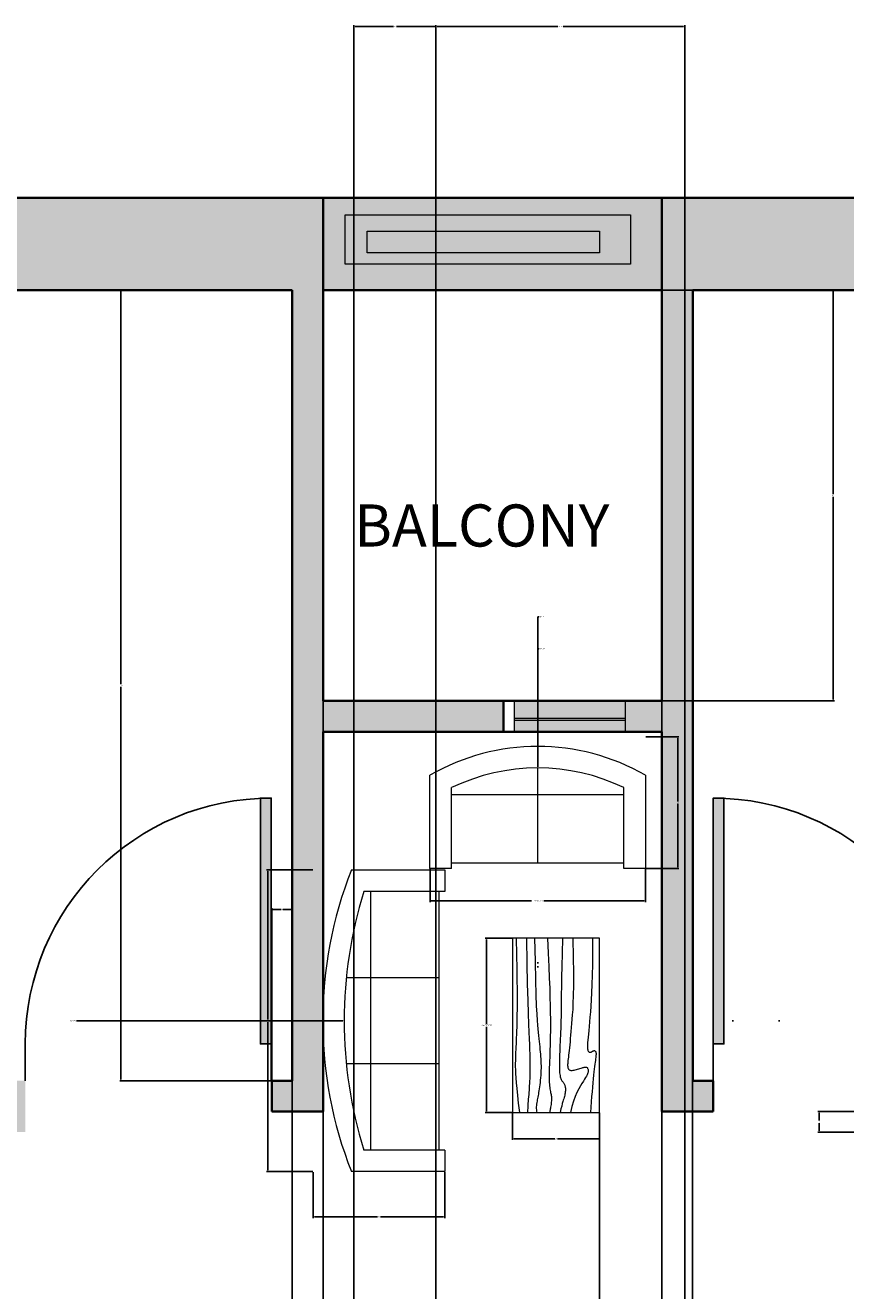
# Model space of a CAD drawing. Units: inches. Extents: x 1434 to 1845, y 1483 to 2014.
# Tile 10 of 11: x 1573 to 1693, y 1829 to 2014. Entities that reach past the tile are written whole.
import ezdxf

# ---------------------------------------------------------------- set-up
doc = ezdxf.new("R2010")
doc.units = ezdxf.units.IN
for name, color, linetype, lineweight in [('A-ANNO-DIMS', 2, 'Continuous', 18), ('A-AREA-IDEN', 7, 'Continuous', 25), ('A-DOOR', 3, 'Continuous', 25), ('A-FURN', 9, 'Continuous', 18), ('A-GLAZ', 4, 'Continuous', 18), ('A-GLAZ-PATT', 9, 'Continuous', 13), ('A-WALL', 7, 'Continuous', 35), ('A-WALL-PATT', 8, 'Continuous', 13)]:
    doc.layers.add(name, color=color, linetype=linetype, lineweight=lineweight)
doc.layers.add('A-DOOR-PATT', color=39, linetype='Continuous', lineweight=13, true_color=0x58382b)
doc.styles.get("Standard").update_dxf_attribs({"font": 'arial.ttf'})
doc.dimstyles.get("Standard").update_dxf_attribs({"dimtxt": 0.18, "dimasz": 0.18, "dimexe": 0.18, "dimexo": 0.0625, "dimgap": 0.09, "dimtad": 0, "dimtih": 1, "dimtoh": 1, "dimdec": 4, "dimzin": 0, "dimdsep": 46, "dimtxsty": 'Standard', "dimcen": 0.09, "dimadec": 0, "dimazin": 0, "dimtfac": 1, "dimtdec": 4, "dimtofl": 0, "dimtmove": 0, "dimatfit": 3, "dimfxl": 1, "dimtolj": 1, "dimtzin": 0, "dimarcsym": 0})

# ---------------------------------------------------------------- blocks, each defined once
blk = doc.blocks.new('*U2')
for p, q in [((0, 0), (0, -6)), ((-40, 0), (-40, -6))]:
    blk.add_line(p, q)
blk.add_lwpolyline([(0, 0), (0, 40), (-1.75, 40), (-1.75, 0)], close=True)
blk.add_arc((0, 0), 40, 90, 180)
blk = doc.blocks.new('*U3')
for p, q in [((0, 0), (0, -6)), ((40, 0), (40, -6))]:
    blk.add_line(p, q)
blk.add_lwpolyline([(0, 0), (0, 40), (1.75, 40), (1.75, 0)], close=True)
blk.add_arc((0, 0), 40, 0, 90)
blk = doc.blocks.new('Sofa - Roundback 7 ft.')
for p, q in [((-12.00002, -32.4421), (-12.00003, -6.5971)), ((11.99997, -32.4421), (11.99998, -6.5971)), ((-36.000027, -34), (-36.000027, -11.4696)), ((-35.999844, -13.3819), (35.9998, -13.3819)), ((35.99998, -34), (35.99998, -11.4696)), ((-36.000027, -32.4421), (35.99998, -32.4421))]:
    blk.add_line(p, q)
for points in [[(-36.000027, -34), (-42.000027, -34), (-42.000027, -8)], [(41.99998, -8), (41.99998, -34), (35.99998, -34)]]:
    blk.add_lwpolyline(points)
for centre, radius, start, end in [((0, -114.25), 114.25, 68.43141, 111.5686), ((-0.00001, -127.1968), 121.1968, 72.72033, 107.2797)]:
    blk.add_arc(centre, radius, start, end)
blk = doc.blocks.new('Sofa - Roundback Loveseat 5 ft.')
for p, q in [((0, -32.44198), (0, -5.99998)), ((-24, -33.99998), (-24, -11.46958)), ((-23.9998, -13.38178), (23.99986, -13.38178)), ((24.00004, -33.99998), (24.00004, -11.46958)), ((-24, -32.44198), (24.00004, -32.44198))]:
    blk.add_line(p, q)
for points in [[(-24, -33.99998), (-30, -33.99998), (-30, -7.99998)], [(30.00004, -7.99998), (30.00004, -33.99998), (24.00004, -33.99998)]]:
    blk.add_lwpolyline(points)
for centre, radius, start, end in [((0, -60.24998), 60.24998, 60.13715, 119.8628), ((0, -61.38438), 55.38444, 64.32083, 115.6792)]:
    blk.add_arc(centre, radius, start, end)
blk = doc.blocks.new('Table - Rectangular Woodgrain 60 x 30 in.')
for p, q in [((0, 0), (0, -30)), ((60, 0), (0, 0)), ((60, -30), (60, 0)), ((0, -30), (60, -30))]:
    blk.add_line(p, q)
for points in [[(0, -2.4), (4.8155, -2.418), (9.0302, -2.4688), (12.709, -2.5477), (15.9167, -2.65), (18.7181, -2.7711), (21.1781, -2.9063), (23.3616, -3.0508), (25.3333, -3.2), (27.1477, -3.3495), (28.8172, -3.4958), (30.3437, -3.636), (31.7291, -3.7667), (32.9756, -3.8849), (34.0849, -3.9875), (35.059, -4.0714), (35.9, -4.1334), (36.6114, -4.1711), (37.2041, -4.1854), (37.6906, -4.1779), (38.0833, -4.15), (38.3948, -4.1034), (38.6375, -4.0396), (38.8239, -3.9602), (38.9666, -3.8667), (39.0764, -3.7608), (39.1573, -3.6448), (39.2116, -3.521), (39.2416, -3.3917), (39.2498, -3.2593), (39.2385, -3.1261), (39.21, -2.9944), (39.1666, -2.8667), (39.111, -2.7447), (39.0468, -2.6281), (38.978, -2.5163), (38.9083, -2.4083), (38.8418, -2.3035), (38.7823, -2.201), (38.7337, -2.1001), (38.7, -2), (38.6844, -1.9003), (38.6875, -1.8021), (38.7094, -1.707), (38.75, -1.6167), (38.8094, -1.5326), (38.8875, -1.4563), (38.9844, -1.3893), (39.1, -1.3333), (39.2351, -1.2896), (39.3937, -1.2583), (39.5804, -1.2396), (39.8, -1.2333), (40.057, -1.2396), (40.3562, -1.2583), (40.7023, -1.2896), (41.1, -1.3333), (41.5547, -1.3895), (42.0755, -1.4573), (42.6721, -1.5361), (43.3542, -1.625), (44.1316, -1.7233), (45.014, -1.8302), (46.0114, -1.9449), (47.1333, -2.0667), (48.3862, -2.1947), (49.7625, -2.3281), (51.2513, -2.4663), (52.8416, -2.6083), (54.5226, -2.7535), (56.2833, -2.9011), (58.1127, -3.0501), (60, -3.2)], [(0, -9.2), (6.5759, -9.0858), (11.9385, -9.0365), (16.2527, -9.0418), (19.6833, -9.0917), (22.3952, -9.1759), (24.5531, -9.2844), (26.322, -9.4069), (27.8666, -9.5333), (29.3241, -9.6553), (30.7203, -9.7719), (32.0532, -9.8837), (33.3208, -9.9917), (34.5213, -10.0965), (35.6526, -10.199), (36.7128, -10.2999), (37.7, -10.4), (38.6129, -10.4996), (39.4531, -10.5969), (40.223, -10.6895), (40.925, -10.775), (41.5613, -10.8512), (42.1344, -10.9156), (42.6465, -10.966), (43.1, -11), (43.4976, -11.0158), (43.8437, -11.0136), (44.143, -10.9942), (44.4, -10.9583), (44.6195, -10.9069), (44.8062, -10.8406), (44.9648, -10.7603), (45.1, -10.6667), (45.2155, -10.5598), (45.3114, -10.4365), (45.3871, -10.2929), (45.4416, -10.125), (45.4743, -9.929), (45.4844, -9.7011), (45.4709, -9.4371), (45.4333, -9.1333), (45.3716, -8.7883), (45.2896, -8.4104), (45.1919, -8.0107), (45.0833, -7.6), (44.9685, -7.1893), (44.8521, -6.7896), (44.7388, -6.4117), (44.6333, -6.0667), (44.54, -5.7628), (44.4614, -5.4979), (44.4001, -5.2675), (44.3583, -5.0667), (44.3384, -4.8909), (44.3427, -4.7354), (44.3736, -4.5956), (44.4333, -4.4667), (44.5236, -4.3453), (44.6427, -4.2333), (44.7884, -4.1339), (44.9583, -4.05), (45.1501, -3.9849), (45.3614, -3.9417), (45.59, -3.9234), (45.8333, -3.9333), (46.0915, -3.9749), (46.3734, -4.0531), (46.6906, -4.1736), (47.0542, -4.3417), (47.4756, -4.5629), (47.9661, -4.8427), (48.5372, -5.1866), (49.2, -5.6), (49.9676, -6.0844), (50.8594, -6.625), (51.8965, -7.2031), (53.1, -7.8), (54.491, -8.3969), (56.0906, -8.975), (57.9199, -9.5156), (60, -10)], [(0, -12.8), (5.1847, -12.9322), (9.6213, -13.0323), (13.3963, -13.1059), (16.5958, -13.1583), (19.3063, -13.1952), (21.614, -13.2219), (23.6054, -13.2439), (25.3666, -13.2667), (26.9728, -13.2947), (28.4531, -13.3281), (29.8256, -13.3663), (31.1083, -13.4083), (32.3191, -13.4535), (33.476, -13.501), (34.597, -13.5501), (35.7, -13.6), (36.7984, -13.6497), (37.8875, -13.6979), (38.9578, -13.743), (40, -13.7833), (41.0047, -13.8174), (41.9625, -13.8438), (42.864, -13.8607), (43.7, -13.8667), (44.4631, -13.8604), (45.1552, -13.8417), (45.7801, -13.8104), (46.3416, -13.7667), (46.8439, -13.7104), (47.2906, -13.6417), (47.6858, -13.5604), (48.0333, -13.4667), (48.3375, -13.3608), (48.6042, -13.2448), (48.8396, -13.121), (49.05, -12.9917), (49.2417, -12.8593), (49.4208, -12.7261), (49.5937, -12.5944), (49.7667, -12.4667), (49.9452, -12.3451), (50.1323, -12.2313), (50.3303, -12.1268), (50.5416, -12.0333), (50.7686, -11.9524), (51.0135, -11.8854), (51.2788, -11.8341), (51.5666, -11.8), (51.8785, -11.7843), (52.2116, -11.7865), (52.562, -11.8059), (52.926, -11.8417), (53.2998, -11.8931), (53.6795, -11.9594), (54.0614, -12.0397), (54.4416, -12.1333), (54.8223, -12.2401), (55.2293, -12.3625), (55.6942, -12.5037), (56.2489, -12.6667), (56.9251, -12.8547), (57.7545, -13.0708), (58.7689, -13.3182), (60, -13.6)], [(0, -18), (5.124, -17.7273), (9.6609, -17.5057), (13.6705, -17.3303), (17.2125, -17.1958), (20.3467, -17.0973), (23.1328, -17.0297), (25.6307, -16.9878), (27.9, -16.9667), (29.9928, -16.9617), (31.9302, -16.9703), (33.7254, -16.9907), (35.3917, -17.0208), (36.9423, -17.0588), (38.3906, -17.1026), (39.7499, -17.1503), (41.0333, -17.2), (42.2519, -17.2496), (43.4073, -17.2969), (44.4986, -17.3395), (45.525, -17.375), (46.4858, -17.4012), (47.3802, -17.4156), (48.2074, -17.416), (48.9667, -17.4), (49.6583, -17.3662), (50.2872, -17.3167), (50.8595, -17.2547), (51.3812, -17.1833), (51.8584, -17.1057), (52.2971, -17.025), (52.7034, -16.9443), (53.0833, -16.8667), (53.443, -16.7951), (53.789, -16.7313), (54.128, -16.6768), (54.4666, -16.6334), (54.8115, -16.6024), (55.1693, -16.5854), (55.5465, -16.5841), (55.95, -16.6), (56.3828, -16.6337), (56.8346, -16.6823), (57.2915, -16.7418), (57.7396, -16.8084), (58.165, -16.878), (58.5539, -16.9469), (58.8924, -17.0111), (59.1666, -17.0667), (59.3679, -17.1107), (59.5078, -17.1438), (59.6032, -17.1675), (59.6708, -17.1833), (59.7275, -17.193), (59.7901, -17.1979), (59.8753, -17.1998), (60, -17.2)], [(0, -22.4), (8.0098, -22.2501), (14.4094, -22.1011), (19.4168, -21.9535), (23.25, -21.8083), (26.1269, -21.6663), (28.2656, -21.5281), (29.884, -21.3947), (31.2, -21.2667), (32.3967, -21.1448), (33.5172, -21.0292), (34.5697, -20.9198), (35.5625, -20.8167), (36.5037, -20.7198), (37.4015, -20.6292), (38.2642, -20.5448), (39.1, -20.4667), (39.9164, -20.3951), (40.7187, -20.3313), (41.5117, -20.2768), (42.3, -20.2333), (43.0883, -20.2024), (43.8812, -20.1854), (44.6836, -20.1841), (45.5, -20.2), (46.3328, -20.234), (47.1747, -20.2844), (48.0163, -20.3488), (48.8479, -20.425), (49.66, -20.5106), (50.4429, -20.6031), (51.1872, -20.7004), (51.8833, -20.8), (52.5246, -20.8999), (53.1166, -20.9995), (53.6681, -21.0983), (54.1875, -21.1958), (54.6834, -21.2919), (55.1646, -21.3859), (55.6394, -21.4777), (56.1167, -21.5667), (56.6028, -21.6515), (57.0961, -21.7266), (57.5929, -21.7852), (58.0896, -21.8208), (58.5823, -21.8268), (59.0674, -21.7964), (59.5412, -21.723), (60, -21.6)], [(0, -25.2), (8.6355, -25.0504), (15.7026, -24.9031), (21.4049, -24.7606), (25.9458, -24.625), (29.529, -24.4988), (32.3578, -24.3844), (34.6359, -24.284), (36.5667, -24.2), (38.3213, -24.1341), (39.9417, -24.0854), (41.437, -24.0523), (42.8167, -24.0333), (44.0901, -24.0268), (45.2667, -24.0313), (46.3557, -24.0451), (47.3667, -24.0667), (48.309, -24.0947), (49.1928, -24.1287), (50.0284, -24.168), (50.826, -24.2125), (51.5959, -24.2617), (52.3483, -24.3151), (53.0935, -24.3725), (53.8417, -24.4334), (54.6009, -24.497), (55.3699, -24.561), (56.1454, -24.6226), (56.9239, -24.6792), (57.7021, -24.7279), (58.4764, -24.7662), (59.2435, -24.7911), (60, -24.8)], [(0, -28.8), (5.6867, -28.6681), (10.45, -28.5698), (14.407, -28.5012), (17.675, -28.4584), (20.3711, -28.4374), (22.6125, -28.4344), (24.5164, -28.4455), (26.2, -28.4667), (27.762, -28.4947), (29.2276, -28.5281), (30.6033, -28.5663), (31.8958, -28.6084), (33.1118, -28.6535), (34.2578, -28.7011), (35.3405, -28.7501), (36.3666, -28.8), (37.3443, -28.8497), (38.288, -28.8974), (39.2137, -28.9412), (40.1375, -28.9792), (41.0753, -29.0093), (42.0432, -29.0297), (43.0572, -29.0384), (44.1333, -29.0333), (45.2936, -29.0114), (46.5843, -28.9641), (48.0579, -28.8816), (49.7666, -28.7542), (51.7629, -28.5721), (54.0989, -28.3255), (56.8272, -28.0048), (60, -27.6)]]:
    blk.add_lwpolyline(points)
blk = doc.blocks.new('*D38')
at = {"layer": 'A-ANNO-DIMS', "color": 0, "lineweight": -2, "transparency": 16777216}
for p, q in [((1615.46, 1890.16), (1608.73, 1890.16)), ((1608.91, 1889.98), (1608.91, 1868.31)), ((1608.91, 1846.28), (1608.91, 1867.94)), ((1615.46, 1846.1), (1608.73, 1846.1))]:
    blk.add_line(p, q, dxfattribs=at)
at = {"layer": 'A-ANNO-DIMS', "color": 0, "transparency": 16777216}
for points in [[(1608.88, 1889.98), (1608.94, 1889.98), (1608.91, 1890.16)], [(1608.88, 1846.28), (1608.94, 1846.28), (1608.91, 1846.1)]]:
    blk.add_solid(points, dxfattribs=at)
at = {"layer": 'Defpoints', "color": 0, "transparency": 16777216}
for p in [(1608.91, 1890.16), (1615.52, 1890.16), (1615.52, 1846.1)]:
    blk.add_point(p, dxfattribs=at)
at = {"layer": 'A-ANNO-DIMS', "color": 0, "transparency": 16777216, "insert": (1608.91, 1868.13), "char_height": 0.18, "attachment_point": 5}
blk.add_mtext('\\A1;SOFA 44', dxfattribs=at)
blk = doc.blocks.new('*D39')
at = {"layer": 'A-ANNO-DIMS', "color": 0, "lineweight": -2, "transparency": 16777216}
for p, q in [((1615.52, 1846.03), (1615.52, 1839.31)), ((1634.75, 1846.03), (1634.75, 1839.31)), ((1615.7, 1839.49), (1624.92, 1839.49)), ((1634.57, 1839.49), (1625.35, 1839.49))]:
    blk.add_line(p, q, dxfattribs=at)
at = {"layer": 'A-ANNO-DIMS', "color": 0, "transparency": 16777216}
for points in [[(1615.7, 1839.52), (1615.7, 1839.46), (1615.52, 1839.49)], [(1634.57, 1839.52), (1634.57, 1839.46), (1634.75, 1839.49)]]:
    blk.add_solid(points, dxfattribs=at)
at = {"layer": 'Defpoints', "color": 0, "transparency": 16777216}
for p in [(1615.52, 1846.1), (1634.75, 1846.1), (1615.52, 1839.49)]:
    blk.add_point(p, dxfattribs=at)
at = {"layer": 'A-ANNO-DIMS', "color": 0, "transparency": 16777216, "insert": (1625.13, 1839.49), "char_height": 0.18, "attachment_point": 5}
blk.add_mtext('\\A1;19', dxfattribs=at)
blk = doc.blocks.new('*D40')
at = {"layer": 'A-ANNO-DIMS', "color": 0, "lineweight": -2, "transparency": 16777216}
for p, q in [((1632.6, 1890.31), (1632.6, 1885.47)), ((1664.07, 1890.31), (1664.07, 1885.47)), ((1632.78, 1885.65), (1647.44, 1885.65)), ((1663.89, 1885.65), (1649.23, 1885.65))]:
    blk.add_line(p, q, dxfattribs=at)
at = {"layer": 'A-ANNO-DIMS', "color": 0, "transparency": 16777216}
for points in [[(1632.78, 1885.68), (1632.78, 1885.62), (1632.6, 1885.65)], [(1663.89, 1885.68), (1663.89, 1885.62), (1664.07, 1885.65)]]:
    blk.add_solid(points, dxfattribs=at)
at = {"layer": 'Defpoints', "color": 0, "transparency": 16777216}
for p in [(1632.6, 1890.37), (1664.07, 1890.37), (1664.07, 1885.65)]:
    blk.add_point(p, dxfattribs=at)
at = {"layer": 'A-ANNO-DIMS', "color": 0, "transparency": 16777216, "insert": (1648.33, 1885.65), "char_height": 0.18, "attachment_point": 5}
blk.add_mtext('\\A1;LOVESEAT 31', dxfattribs=at)
blk = doc.blocks.new('*D41')
at = {"layer": 'A-ANNO-DIMS', "color": 0, "lineweight": -2, "transparency": 16777216}
for p, q in [((1664.13, 1909.6), (1668.97, 1909.6)), ((1668.79, 1909.42), (1668.79, 1900.17)), ((1668.79, 1890.55), (1668.79, 1899.8)), ((1664.13, 1890.37), (1668.97, 1890.37))]:
    blk.add_line(p, q, dxfattribs=at)
at = {"layer": 'A-ANNO-DIMS', "color": 0, "transparency": 16777216}
for points in [[(1668.76, 1909.42), (1668.82, 1909.42), (1668.79, 1909.6)], [(1668.76, 1890.55), (1668.82, 1890.55), (1668.79, 1890.37)]]:
    blk.add_solid(points, dxfattribs=at)
at = {"layer": 'Defpoints', "color": 0, "transparency": 16777216}
for p in [(1664.07, 1909.6), (1668.79, 1909.6), (1664.07, 1890.37)]:
    blk.add_point(p, dxfattribs=at)
at = {"layer": 'A-ANNO-DIMS', "color": 0, "transparency": 16777216, "insert": (1668.79, 1899.99), "char_height": 0.18, "attachment_point": 5}
blk.add_mtext('\\A1;19', dxfattribs=at)
blk = doc.blocks.new('*D44')
at = {"layer": 'A-ANNO-DIMS', "color": 0, "lineweight": -2, "transparency": 16777216}
for p, q in [((1644.59, 1880.17), (1640.66, 1880.17)), ((1640.84, 1879.99), (1640.84, 1867.63)), ((1640.84, 1854.9), (1640.84, 1867.26)), ((1644.59, 1854.72), (1640.66, 1854.72))]:
    blk.add_line(p, q, dxfattribs=at)
at = {"layer": 'A-ANNO-DIMS', "color": 0, "transparency": 16777216}
for points in [[(1640.81, 1879.99), (1640.87, 1879.99), (1640.84, 1880.17)], [(1640.81, 1854.9), (1640.87, 1854.9), (1640.84, 1854.72)]]:
    blk.add_solid(points, dxfattribs=at)
at = {"layer": 'Defpoints', "color": 0, "transparency": 16777216}
for p in [(1644.65, 1880.17), (1640.84, 1854.72), (1644.65, 1854.72)]:
    blk.add_point(p, dxfattribs=at)
at = {"layer": 'A-ANNO-DIMS', "color": 0, "transparency": 16777216, "insert": (1640.84, 1867.45), "char_height": 0.18, "attachment_point": 5}
blk.add_mtext('\\A1;LOW TABLE 25', dxfattribs=at)
blk = doc.blocks.new('*D45')
at = {"layer": 'A-ANNO-DIMS', "color": 0, "lineweight": -2, "transparency": 16777216}
for p, q in [((1644.65, 1854.66), (1644.65, 1850.72)), ((1657.38, 1854.66), (1657.38, 1850.72)), ((1644.83, 1850.9), (1650.81, 1850.9)), ((1657.2, 1850.9), (1651.23, 1850.9))]:
    blk.add_line(p, q, dxfattribs=at)
at = {"layer": 'A-ANNO-DIMS', "color": 0, "transparency": 16777216}
for points in [[(1644.83, 1850.93), (1644.83, 1850.87), (1644.65, 1850.9)], [(1657.2, 1850.93), (1657.2, 1850.87), (1657.38, 1850.9)]]:
    blk.add_solid(points, dxfattribs=at)
at = {"layer": 'Defpoints', "color": 0, "transparency": 16777216}
for p in [(1644.65, 1854.72), (1657.38, 1854.72), (1657.38, 1850.9)]:
    blk.add_point(p, dxfattribs=at)
at = {"layer": 'A-ANNO-DIMS', "color": 0, "transparency": 16777216, "insert": (1651.02, 1850.9), "char_height": 0.18, "attachment_point": 5}
blk.add_mtext('\\A1;13', dxfattribs=at)
blk = doc.blocks.new('*D56')
at = {"layer": 'A-ANNO-DIMS', "color": 0, "lineweight": -2, "transparency": 16777216}
for p, q in [((1472.97, 1974.79), (1472.97, 1483.15)), ((1612.47, 1974.79), (1612.47, 1483.15)), ((1473.15, 1483.33), (1542.34, 1483.33)), ((1612.29, 1483.33), (1543.11, 1483.33))]:
    blk.add_line(p, q, dxfattribs=at)
at = {"layer": 'A-ANNO-DIMS', "color": 0, "transparency": 16777216}
for points in [[(1473.15, 1483.36), (1473.15, 1483.3), (1472.97, 1483.33)], [(1612.29, 1483.36), (1612.29, 1483.3), (1612.47, 1483.33)]]:
    blk.add_solid(points, dxfattribs=at)
at = {"layer": 'Defpoints', "color": 0, "transparency": 16777216}
for p in [(1472.97, 1974.86), (1612.47, 1974.86), (1612.47, 1483.33)]:
    blk.add_point(p, dxfattribs=at)
at = {"layer": 'A-ANNO-DIMS', "color": 0, "transparency": 16777216, "insert": (1542.72, 1483.33), "char_height": 0.18, "attachment_point": 5}
blk.add_mtext('\\A1;139.5', dxfattribs=at)
blk = doc.blocks.new('*D57')
at = {"layer": 'A-ANNO-DIMS', "color": 0, "lineweight": -2, "transparency": 16777216}
for p, q in [((1616.97, 1974.79), (1616.97, 1483.15)), ((1666.47, 1974.79), (1666.47, 1483.15)), ((1617.15, 1483.33), (1641.4, 1483.33)), ((1666.29, 1483.33), (1642.05, 1483.33))]:
    blk.add_line(p, q, dxfattribs=at)
at = {"layer": 'A-ANNO-DIMS', "color": 0, "transparency": 16777216}
for points in [[(1617.15, 1483.36), (1617.15, 1483.3), (1616.97, 1483.33)], [(1666.29, 1483.36), (1666.29, 1483.3), (1666.47, 1483.33)]]:
    blk.add_solid(points, dxfattribs=at)
at = {"layer": 'Defpoints', "color": 0, "transparency": 16777216}
for p in [(1616.97, 1974.86), (1666.47, 1974.86), (1666.47, 1483.33)]:
    blk.add_point(p, dxfattribs=at)
at = {"layer": 'A-ANNO-DIMS', "color": 0, "transparency": 16777216, "insert": (1641.72, 1483.33), "char_height": 0.18, "attachment_point": 5}
blk.add_mtext('\\A1;49.5', dxfattribs=at)
blk = doc.blocks.new('*D58')
at = {"layer": 'A-ANNO-DIMS', "color": 0, "lineweight": -2, "transparency": 16777216}
for p, q in [((1670.97, 1974.79), (1670.97, 1483.15)), ((1810.47, 1974.79), (1810.47, 1483.15)), ((1671.15, 1483.33), (1740.34, 1483.33)), ((1810.29, 1483.33), (1741.11, 1483.33))]:
    blk.add_line(p, q, dxfattribs=at)
at = {"layer": 'A-ANNO-DIMS', "color": 0, "transparency": 16777216}
for points in [[(1671.15, 1483.36), (1671.15, 1483.3), (1670.97, 1483.33)], [(1810.29, 1483.36), (1810.29, 1483.3), (1810.47, 1483.33)]]:
    blk.add_solid(points, dxfattribs=at)
at = {"layer": 'Defpoints', "color": 0, "transparency": 16777216}
for p in [(1670.97, 1974.86), (1810.47, 1974.86), (1810.47, 1483.33)]:
    blk.add_point(p, dxfattribs=at)
at = {"layer": 'A-ANNO-DIMS', "color": 0, "transparency": 16777216, "insert": (1740.72, 1483.33), "char_height": 0.18, "attachment_point": 5}
blk.add_mtext('\\A1;139.5', dxfattribs=at)
blk = doc.blocks.new('*D59')
at = {"layer": 'A-ANNO-DIMS', "color": 0, "lineweight": -2, "transparency": 16777216}
for p, q in [((1612.41, 1974.86), (1587.27, 1974.86)), ((1587.45, 1974.68), (1587.45, 1917.29)), ((1587.45, 1859.54), (1587.45, 1916.92)), ((1612.41, 1859.36), (1587.27, 1859.36))]:
    blk.add_line(p, q, dxfattribs=at)
at = {"layer": 'A-ANNO-DIMS', "color": 0, "transparency": 16777216}
for points in [[(1587.42, 1974.68), (1587.48, 1974.68), (1587.45, 1974.86)], [(1587.42, 1859.54), (1587.48, 1859.54), (1587.45, 1859.36)]]:
    blk.add_solid(points, dxfattribs=at)
at = {"layer": 'Defpoints', "color": 0, "transparency": 16777216}
for p in [(1587.45, 1974.86), (1612.47, 1974.86), (1612.47, 1859.36)]:
    blk.add_point(p, dxfattribs=at)
at = {"layer": 'A-ANNO-DIMS', "color": 0, "transparency": 16777216, "insert": (1587.45, 1917.11), "char_height": 0.18, "attachment_point": 5}
blk.add_mtext('\\A1;115.5', dxfattribs=at)
blk = doc.blocks.new('*D60')
at = {"layer": 'A-ANNO-DIMS', "color": 0, "lineweight": -2, "transparency": 16777216}
for p, q in [((1666.54, 1974.86), (1691.68, 1974.86)), ((1691.5, 1974.68), (1691.5, 1945.04)), ((1691.5, 1915.04), (1691.5, 1944.67)), ((1666.54, 1914.86), (1691.68, 1914.86))]:
    blk.add_line(p, q, dxfattribs=at)
at = {"layer": 'A-ANNO-DIMS', "color": 0, "transparency": 16777216}
for points in [[(1691.47, 1974.68), (1691.53, 1974.68), (1691.5, 1974.86)], [(1691.47, 1915.04), (1691.53, 1915.04), (1691.5, 1914.86)]]:
    blk.add_solid(points, dxfattribs=at)
at = {"layer": 'Defpoints', "color": 0, "transparency": 16777216}
for p in [(1666.47, 1974.86), (1666.47, 1914.86), (1691.5, 1914.86)]:
    blk.add_point(p, dxfattribs=at)
at = {"layer": 'A-ANNO-DIMS', "color": 0, "transparency": 16777216, "insert": (1691.5, 1944.86), "char_height": 0.18, "attachment_point": 5}
blk.add_mtext('\\A1;60', dxfattribs=at)
blk = doc.blocks.new('*D71')
at = {"layer": 'A-ANNO-DIMS', "color": 0, "lineweight": -2, "transparency": 16777216}
for p, q in [((1633.47, 1508.42), (1633.47, 2013.56)), ((1633.65, 2013.38), (1651.25, 2013.38)), ((1669.64, 2013.38), (1652.04, 2013.38)), ((1669.82, 1508.42), (1669.82, 2013.56))]:
    blk.add_line(p, q, dxfattribs=at)
at = {"layer": 'A-ANNO-DIMS', "color": 0, "transparency": 16777216}
for points in [[(1633.65, 2013.41), (1633.65, 2013.35), (1633.47, 2013.38)], [(1669.64, 2013.41), (1669.64, 2013.35), (1669.82, 2013.38)]]:
    blk.add_solid(points, dxfattribs=at)
at = {"layer": 'Defpoints', "color": 0, "transparency": 16777216}
for p in [(1669.82, 2013.38), (1633.47, 1508.36), (1669.82, 1508.36)]:
    blk.add_point(p, dxfattribs=at)
at = {"layer": 'A-ANNO-DIMS', "color": 0, "transparency": 16777216, "insert": (1651.65, 2013.38), "char_height": 0.18, "attachment_point": 5}
blk.add_mtext('\\A1;36.35', dxfattribs=at)
blk = doc.blocks.new('*D72')
at = {"layer": 'A-ANNO-DIMS', "color": 0, "lineweight": -2, "transparency": 16777216}
for p, q in [((1621.47, 1517.42), (1621.47, 2013.56)), ((1621.65, 2013.38), (1627.26, 2013.38)), ((1633.29, 2013.38), (1627.68, 2013.38)), ((1633.47, 1517.42), (1633.47, 2013.56))]:
    blk.add_line(p, q, dxfattribs=at)
at = {"layer": 'A-ANNO-DIMS', "color": 0, "transparency": 16777216}
for points in [[(1621.65, 2013.41), (1621.65, 2013.35), (1621.47, 2013.38)], [(1633.29, 2013.41), (1633.29, 2013.35), (1633.47, 2013.38)]]:
    blk.add_solid(points, dxfattribs=at)
at = {"layer": 'Defpoints', "color": 0, "transparency": 16777216}
for p in [(1633.47, 2013.38), (1621.47, 1517.36), (1633.47, 1517.36)]:
    blk.add_point(p, dxfattribs=at)
at = {"layer": 'A-ANNO-DIMS', "color": 0, "transparency": 16777216, "insert": (1627.47, 2013.38), "char_height": 0.18, "attachment_point": 5}
blk.add_mtext('\\A1;12', dxfattribs=at)
blk = doc.blocks.new('*D86')
at = {"layer": 'A-ANNO-DIMS', "color": 0, "lineweight": -2, "transparency": 16777216}
for p, q in [((1657.38, 1854.66), (1657.38, 1483.15)), ((1666.47, 1854.79), (1666.47, 1483.15)), ((1657.56, 1483.33), (1661.53, 1483.33)), ((1666.29, 1483.33), (1662.32, 1483.33))]:
    blk.add_line(p, q, dxfattribs=at)
at = {"layer": 'A-ANNO-DIMS', "color": 0, "transparency": 16777216}
for points in [[(1657.56, 1483.36), (1657.56, 1483.3), (1657.38, 1483.33)], [(1666.29, 1483.36), (1666.29, 1483.3), (1666.47, 1483.33)]]:
    blk.add_solid(points, dxfattribs=at)
at = {"layer": 'Defpoints', "color": 0, "transparency": 16777216}
for p in [(1657.38, 1854.72), (1666.47, 1854.86), (1657.38, 1483.33)]:
    blk.add_point(p, dxfattribs=at)
at = {"layer": 'A-ANNO-DIMS', "color": 0, "transparency": 16777216, "insert": (1661.93, 1483.33), "char_height": 0.18, "attachment_point": 5}
blk.add_mtext('\\A1;9.096', dxfattribs=at)
blk = doc.blocks.new('*D89')
at = {"layer": 'A-ANNO-DIMS', "color": 0, "lineweight": -2, "transparency": 16777216}
for p, q in [((1609.47, 1859.42), (1609.47, 1884.56)), ((1609.65, 1884.38), (1610.83, 1884.38)), ((1612.29, 1884.38), (1611.12, 1884.38)), ((1612.47, 1859.42), (1612.47, 1884.56))]:
    blk.add_line(p, q, dxfattribs=at)
at = {"layer": 'A-ANNO-DIMS', "color": 0, "transparency": 16777216}
for points in [[(1609.65, 1884.41), (1609.65, 1884.35), (1609.47, 1884.38)], [(1612.29, 1884.41), (1612.29, 1884.35), (1612.47, 1884.38)]]:
    blk.add_solid(points, dxfattribs=at)
at = {"layer": 'Defpoints', "color": 0, "transparency": 16777216}
for p in [(1612.47, 1884.38), (1609.47, 1859.36), (1612.47, 1859.36)]:
    blk.add_point(p, dxfattribs=at)
at = {"layer": 'A-ANNO-DIMS', "color": 0, "transparency": 16777216, "insert": (1610.97, 1884.38), "char_height": 0.18, "attachment_point": 5}
blk.add_mtext('\\A1;3', dxfattribs=at)
blk = doc.blocks.new('*D90')
at = {"layer": 'A-ANNO-DIMS', "color": 0, "lineweight": -2, "transparency": 16777216}
for p, q in [((1714.41, 1854.86), (1689.27, 1854.86)), ((1689.45, 1854.68), (1689.45, 1853.54)), ((1689.45, 1852.04), (1689.45, 1853.17)), ((1714.41, 1851.86), (1689.27, 1851.86))]:
    blk.add_line(p, q, dxfattribs=at)
at = {"layer": 'A-ANNO-DIMS', "color": 0, "transparency": 16777216}
for points in [[(1689.42, 1854.68), (1689.48, 1854.68), (1689.45, 1854.86)], [(1689.42, 1852.04), (1689.48, 1852.04), (1689.45, 1851.86)]]:
    blk.add_solid(points, dxfattribs=at)
at = {"layer": 'Defpoints', "color": 0, "transparency": 16777216}
for p in [(1689.45, 1854.86), (1714.47, 1854.86), (1714.47, 1851.86)]:
    blk.add_point(p, dxfattribs=at)
at = {"layer": 'A-ANNO-DIMS', "color": 0, "transparency": 16777216, "insert": (1689.45, 1853.36), "char_height": 0.18, "attachment_point": 5}
blk.add_mtext('\\A1;3', dxfattribs=at)
blk = doc.blocks.new('*D92')
at = {"layer": 'A-ANNO-DIMS', "color": 0, "lineweight": -2, "transparency": 16777216}
for p, q in [((1581.92, 1868.13), (1619.88, 1868.13)), ((1683.54, 1868.13), (1683.72, 1868.13)), ((1683.63, 1868.04), (1683.63, 1868.22))]:
    blk.add_line(p, q, dxfattribs=at)
at = {"layer": 'A-ANNO-DIMS', "color": 0, "transparency": 16777216}
blk.add_solid([(1619.88, 1868.16), (1619.88, 1868.1), (1620.06, 1868.13)], dxfattribs=at)
at = {"layer": 'Defpoints', "color": 0, "transparency": 16777216}
for p in [(1620.06, 1868.13), (1683.63, 1868.13)]:
    blk.add_point(p, dxfattribs=at)
at = {"layer": 'A-ANNO-DIMS', "color": 0, "transparency": 16777216, "insert": (1581.44, 1868.13), "char_height": 0.18, "attachment_point": 5}
blk.add_mtext('\\A1;R63.57', dxfattribs=at)
blk = doc.blocks.new('*D93')
at = {"layer": 'A-ANNO-DIMS', "color": 0, "lineweight": -2, "transparency": 16777216}
for p, q in [((1580.96, 1868.13), (1616.74, 1868.13)), ((1676.75, 1868.13), (1676.93, 1868.13)), ((1676.84, 1868.04), (1676.84, 1868.22))]:
    blk.add_line(p, q, dxfattribs=at)
at = {"layer": 'A-ANNO-DIMS', "color": 0, "transparency": 16777216}
blk.add_solid([(1616.74, 1868.16), (1616.74, 1868.1), (1616.92, 1868.13)], dxfattribs=at)
at = {"layer": 'Defpoints', "color": 0, "transparency": 16777216}
for p in [(1616.92, 1868.13), (1676.84, 1868.13)]:
    blk.add_point(p, dxfattribs=at)
at = {"layer": 'A-ANNO-DIMS', "color": 0, "transparency": 16777216, "insert": (1580.48, 1868.13), "char_height": 0.18, "attachment_point": 5}
blk.add_mtext('\\A1;R59.92', dxfattribs=at)
blk = doc.blocks.new('*D94')
at = {"layer": 'A-ANNO-DIMS', "color": 0, "lineweight": -2, "transparency": 16777216}
for p, q in [((1648.51, 1927.16), (1648.33, 1927.16)), ((1648.33, 1927.16), (1648.33, 1908.38)), ((1648.24, 1876.6), (1648.42, 1876.6)), ((1648.33, 1876.51), (1648.33, 1876.69))]:
    blk.add_line(p, q, dxfattribs=at)
at = {"layer": 'A-ANNO-DIMS', "color": 0, "transparency": 16777216}
blk.add_solid([(1648.3, 1908.38), (1648.36, 1908.38), (1648.33, 1908.2)], dxfattribs=at)
at = {"layer": 'Defpoints', "color": 0, "transparency": 16777216}
for p in [(1648.33, 1908.2), (1648.33, 1876.6)]:
    blk.add_point(p, dxfattribs=at)
at = {"layer": 'A-ANNO-DIMS', "color": 0, "transparency": 16777216, "insert": (1648.92, 1927.16), "char_height": 0.18, "attachment_point": 5}
blk.add_mtext('\\A1;R31.6', dxfattribs=at)
blk = doc.blocks.new('*D95')
at = {"layer": 'A-ANNO-DIMS', "color": 0, "lineweight": -2, "transparency": 16777216}
for p, q in [((1648.51, 1922.48), (1648.33, 1922.48)), ((1648.33, 1922.48), (1648.33, 1905.24)), ((1648.24, 1876.01), (1648.42, 1876.01)), ((1648.33, 1875.92), (1648.33, 1876.1))]:
    blk.add_line(p, q, dxfattribs=at)
at = {"layer": 'A-ANNO-DIMS', "color": 0, "transparency": 16777216}
blk.add_solid([(1648.3, 1905.24), (1648.36, 1905.24), (1648.33, 1905.06)], dxfattribs=at)
at = {"layer": 'Defpoints', "color": 0, "transparency": 16777216}
for p in [(1648.33, 1905.06), (1648.33, 1876.01)]:
    blk.add_point(p, dxfattribs=at)
at = {"layer": 'A-ANNO-DIMS', "color": 0, "transparency": 16777216, "insert": (1648.99, 1922.48), "char_height": 0.18, "attachment_point": 5}
blk.add_mtext('\\A1;R29.05', dxfattribs=at)

msp = doc.modelspace()

# ---------------------------------------------------------------- hatches: boundary and pattern name
at = {"layer": 'A-DOOR-PATT'}
h = msp.add_hatch(color=256, dxfattribs=at)
h.dxf.hatch_style = 1
h.paths.add_polyline_path([(1611.5864, 1583.2737), (1575.6681, 1583.2737, 0.01094143), (1575.7025, 1581.7022), (1611.5864, 1581.7022)])
h.paths.add_polyline_path([(1621.4742, 1547.3553), (1616.9742, 1547.3553), (1616.9742, 1544.3553), (1621.4742, 1544.3553)])
h.paths.add_polyline_path([(1635.0456, 1558.627, 0.01094143), (1633.4742, 1558.6614), (1633.4742, 1522.7431), (1635.0456, 1522.7431)])
h.paths.add_polyline_path([(1633.4742, 1517.3553), (1630.4742, 1517.3553), (1630.4742, 1508.3553), (1633.4742, 1508.3553)])
h.paths.add_polyline_path([(1672.8212, 1517.3553), (1669.8212, 1517.3553), (1669.8212, 1508.3553), (1672.8212, 1508.3553)])
h.paths.add_polyline_path([(1613.8925, 1724.9676), (1612.3211, 1724.9676), (1612.3211, 1689.0836, 0.01094143), (1613.8925, 1689.0492)])
h.paths.add_polyline_path([(1789.3925, 1684.9726), (1753.4742, 1684.9726), (1753.4742, 1683.4011), (1789.3925, 1683.4011)])
h.paths.add_polyline_path([(1792.4742, 1679.5848), (1789.4742, 1679.5848), (1789.4742, 1675.0848), (1792.4742, 1675.0848)])
h.paths.add_polyline_path([(1563.5864, 1851.7737), (1527.6681, 1851.7737, 0.01094143), (1527.7025, 1850.2022), (1563.5864, 1850.2022)])
h.paths.add_polyline_path([(1609.3925, 1900.6614, 0.01094143), (1607.8211, 1900.627), (1607.8211, 1864.7431), (1609.3925, 1864.7431)])
h.paths.add_polyline_path([(1675.5456, 1900.627, 0.01094143), (1673.9742, 1900.6614), (1673.9742, 1864.7431), (1675.5456, 1864.7431)])
h.paths.add_polyline_path([(1751.2803, 1851.8553), (1715.3619, 1851.8553), (1715.3619, 1850.2839), (1751.2459, 1850.2839, 0.01094143)])
at = {"layer": 'A-GLAZ-PATT'}
h = msp.add_hatch(color=256, dxfattribs=at)
h.dxf.hatch_style = 1
h.set_gradient(color1=(0, 0, 255), color2=(255, 255, 0), name='SPHERICAL')
h.paths.add_polyline_path([(1666.4742, 1988.3553), (1616.9742, 1988.3553), (1616.9742, 1974.8553), (1666.4742, 1974.8553)])
h.paths.add_polyline_path([(1620.2163, 1978.6438), (1620.2163, 1985.8742), (1661.8944, 1985.8742), (1661.8944, 1978.6438)], flags=16)
h.paths.add_polyline_path([(1623.4137, 1980.3253), (1623.4137, 1983.4641), (1657.3508, 1983.4641), (1657.3508, 1980.3253)], flags=0)
h.paths.add_polyline_path([(1661.8944, 1985.8742), (1620.2163, 1985.8742), (1620.2163, 1978.6438), (1661.8944, 1978.6438)], flags=16)
h = msp.add_hatch(color=256, dxfattribs=at)
h.dxf.hatch_style = 1
h.set_gradient(color1=(0, 0, 255), color2=(255, 255, 0))
h.paths.add_polyline_path([(1661.1087, 1914.8553), (1644.9471, 1914.8553), (1644.9471, 1912.3513), (1661.1087, 1912.3513)])
h.paths.add_polyline_path([(1661.1087, 1912.3513), (1644.9471, 1912.3513), (1644.9471, 1912.0075), (1661.1087, 1912.0075)])
h.paths.add_polyline_path([(1661.1087, 1912.0075), (1644.9471, 1912.0075), (1644.9471, 1910.3553), (1661.1087, 1910.3553)])
at = {"layer": 'A-WALL-PATT'}
h = msp.add_hatch(color=256, dxfattribs=at)
h.dxf.hatch_style = 1
h.paths.add_polyline_path([(1472.9742, 1730.3553), (1577.9742, 1730.3553), (1577.9742, 1734.8553), (1573.4742, 1734.8553), (1573.4742, 1815.8553), (1568.9742, 1815.8553), (1568.9742, 1734.8553), (1472.9742, 1734.8553), (1472.9742, 1770.1951), (1459.9742, 1770.1951), (1459.9742, 1782.1951), (1459.9742, 1818.1951), (1472.9742, 1818.1951), (1472.9742, 1854.8553), (1568.9742, 1854.8553), (1568.9742, 1851.8553), (1573.4742, 1851.8553), (1573.4742, 1854.8553), (1573.4742, 1859.3553), (1472.9742, 1859.3553), (1472.9742, 1899.9369), (1459.9742, 1899.9369), (1459.9742, 1911.9369), (1459.9742, 1947.9369), (1472.9742, 1947.9369), (1472.9742, 1974.8553), (1513.9785, 1974.8553), (1513.9785, 1987.8553), (1561.9785, 1987.8553), (1561.9785, 1974.8553), (1612.4742, 1974.8553), (1612.4742, 1859.3553), (1609.4742, 1859.3553), (1609.4742, 1854.8553), (1616.9742, 1854.8553), (1616.9742, 1910.3553), (1625.153, 1910.3553), (1625.153, 1914.8553), (1616.9742, 1914.8553), (1616.9742, 1988.3553), (1459.4742, 1988.3553), (1459.4742, 1508.3553), (1630.4742, 1508.3553), (1630.4742, 1517.3553), (1472.9742, 1517.3553), (1472.9742, 1586.3553), (1616.9742, 1586.3553), (1616.9742, 1583.3553), (1621.4742, 1583.3553), (1621.4742, 1586.3553), (1621.4742, 1734.8553), (1616.9742, 1734.8553), (1613.9742, 1734.8553), (1613.9742, 1730.3553), (1616.9742, 1730.3553), (1616.9742, 1590.8553), (1472.9742, 1590.8553), (1472.9742, 1635.7299), (1459.9742, 1635.7299), (1459.9742, 1647.7299), (1459.9742, 1683.7299), (1472.9742, 1683.7299)])
h.paths.add_polyline_path([(1819.4742, 1773.1667), (1810.4742, 1773.1667), (1810.4742, 1734.8553), (1714.4742, 1734.8553), (1714.4742, 1815.8553), (1709.9742, 1815.8553), (1709.9742, 1730.3553), (1745.9742, 1730.3553), (1745.9742, 1675.0848), (1753.4742, 1675.0848), (1753.4742, 1679.5848), (1750.4742, 1679.5848), (1750.4742, 1730.3553), (1810.4742, 1730.3553), (1810.4742, 1679.5848), (1792.4742, 1679.5848), (1792.4742, 1675.0848), (1810.4742, 1675.0848), (1810.4742, 1517.3553), (1775.1129, 1517.3553), (1775.1129, 1508.3553), (1819.4742, 1508.3553)])
h.paths.add_polyline_path([(1739.1129, 1517.3553), (1694.9742, 1517.3553), (1694.9742, 1730.3553), (1690.4742, 1730.3553), (1690.4742, 1517.3553), (1678.4742, 1517.3553), (1675.4742, 1517.3553), (1672.8212, 1517.3553), (1672.8212, 1508.3553), (1678.4742, 1508.3553), (1739.1129, 1508.3553)])
h.paths.add_polyline_path([(1735.6549, 1987.8553), (1783.6549, 1987.8553), (1783.6549, 1974.8553), (1810.4742, 1974.8553), (1810.4742, 1859.3553), (1709.9742, 1859.3553), (1709.9742, 1854.8553), (1709.9742, 1851.8553), (1714.4742, 1851.8553), (1714.4742, 1854.8553), (1810.4742, 1854.8553), (1810.4742, 1809.1667), (1819.4742, 1809.1667), (1819.4742, 1988.3553), (1666.4742, 1988.3553), (1666.4742, 1914.8553), (1661.1087, 1914.8553), (1661.1087, 1910.3553), (1666.4742, 1910.3553), (1666.4742, 1854.8553), (1673.9742, 1854.8553), (1673.9742, 1859.3553), (1670.9742, 1859.3553), (1670.9742, 1974.8553), (1735.6549, 1974.8553)])
h = msp.add_hatch(color=256, dxfattribs=at)
h.dxf.hatch_style = 1
h.paths.add_polyline_path([(1643.3107, 1914.8553), (1625.153, 1914.8553), (1625.153, 1910.3553), (1643.3107, 1910.3553)])

# ---------------------------------------------------------------- linework, layer by layer
at = {"layer": 'A-GLAZ'}
for points in [[(1620.2163, 1985.8742), (1661.8944, 1985.8742), (1661.8944, 1978.6438), (1620.2163, 1978.6438)], [(1623.4137, 1983.4641), (1657.3508, 1983.4641), (1657.3508, 1980.3253), (1623.4137, 1980.3253)], [(1644.9471, 1914.8553), (1661.1087, 1914.8553), (1661.1087, 1910.3553), (1644.9471, 1910.3553)], [(1644.9471, 1912.3513), (1661.1087, 1912.3513), (1661.1087, 1912.0075), (1644.9471, 1912.0075)]]:
    msp.add_lwpolyline(points, close=True, dxfattribs=at)
at = {"layer": 'A-WALL'}
for p, q in [((1616.9742, 1988.3553), (1616.9742, 1914.8553)), ((1666.4742, 1914.8553), (1666.4742, 1988.3553)), ((1612.4742, 1974.8553), (1472.9742, 1974.8553)), ((1612.4742, 1974.8553), (1612.4742, 1859.3553)), ((1616.9742, 1974.8553), (1616.9742, 1914.8553)), ((1666.4742, 1974.8553), (1616.9742, 1974.8553)), ((1810.4742, 1974.8553), (1670.9742, 1974.8553)), ((1670.9742, 1859.3553), (1670.9742, 1974.8553)), ((1666.4742, 1914.8553), (1616.9742, 1914.8553)), ((1625.153, 1914.8553), (1643.3107, 1914.8553)), ((1643.3107, 1914.8553), (1643.3107, 1910.3553)), ((1666.4742, 1910.3553), (1616.9742, 1910.3553)), ((1616.9742, 1910.3553), (1616.9742, 1854.8553)), ((1616.9742, 1910.3553), (1616.9742, 1854.8553)), ((1643.3107, 1910.3553), (1625.153, 1910.3553)), ((1666.4742, 1854.8553), (1666.4742, 1910.3553)), ((1612.4742, 1859.3553), (1609.4742, 1859.3553)), ((1609.4742, 1859.3553), (1609.4742, 1854.8553)), ((1673.9742, 1859.3553), (1670.9742, 1859.3553)), ((1673.9742, 1854.8553), (1673.9742, 1859.3553)), ((1616.9742, 1854.8553), (1609.4742, 1854.8553)), ((1673.9742, 1854.8553), (1666.4742, 1854.8553))]:
    msp.add_line(p, q, dxfattribs=at)
msp.add_lwpolyline([(1678.4742, 1508.3553), (1819.4742, 1508.3553), (1819.4742, 1988.3553), (1459.4742, 1988.3553), (1459.4742, 1508.3553), (1630.4742, 1508.3553)], dxfattribs=at)

# ---------------------------------------------------------------- block references
at = {"layer": 'A-DOOR', "xscale": 0.8979587755198419, "yscale": 0.8979587755198419, "zscale": 0.8979587755198419}
for name, p in [('*U2', (1609.3925, 1864.7431)), ('*U3', (1673.9742, 1864.7431))]:
    msp.add_blockref(name, p, dxfattribs=at)
at = {"layer": 'A-FURN', "xscale": 0.5245049688681437, "yscale": 0.5245049688681437, "zscale": 0.5245049688681437}
msp.add_blockref('Sofa - Roundback Loveseat 5 ft.', (1648.332, 1908.2023), dxfattribs=at)
at = {"layer": 'A-FURN'}
for name, p, xscale, yscale, zscale, rotation in [('Sofa - Roundback 7 ft.', (1616.9178, 1868.1263), 0.5245049688681437, 0.5245049688681437, 0.5245049688681437, 90), ('Table - Rectangular Woodgrain 60 x 30 in.', (1657.3781, 1880.1696), 0.4241524324166927, 0.4241524324166927, 0.4241524324166927, 270)]:
    msp.add_blockref(name, p, dxfattribs=dict(at, xscale=xscale, yscale=yscale, zscale=zscale, rotation=rotation))

# ---------------------------------------------------------------- texts
at = {"layer": 'A-AREA-IDEN'}
msp.add_text('BALCONY ', height=6.15089, dxfattribs=at).set_placement((1621.5202, 1937.4089))

# ---------------------------------------------------------------- dimensions: what is measured, and where the dimension line sits
at = {"layer": 'A-ANNO-DIMS'}
for base, p1, p2, override, picture, middle in [((1633.4742, 2013.3803), (1621.4742, 1517.3553), (1633.4742, 1517.3553), {"dimdec": 0, "dimlfac": 1, "dimrnd": 0, "dimzin": 0, "dimdsep": 46, "dimlunit": 2}, '*D72', (1627.4742, 2013.3803)), ((1669.8212, 2013.3803), (1633.4742, 1508.3553), (1669.8212, 1508.3553), {"dimdec": 2, "dimlfac": 1, "dimrnd": 0, "dimzin": 0, "dimdsep": 46, "dimlunit": 2}, '*D71', (1651.6477, 2013.3803)), ((1612.4742, 1483.3303), (1472.9742, 1974.8553), (1612.4742, 1974.8553), {"dimdec": 1, "dimlfac": 1, "dimrnd": 0, "dimzin": 0, "dimdsep": 46, "dimlunit": 2}, '*D56', (1542.7242, 1483.3303)), ((1666.4742, 1483.3303), (1616.9742, 1974.8553), (1666.4742, 1974.8553), {"dimdec": 1, "dimlfac": 1, "dimrnd": 0, "dimzin": 0, "dimdsep": 46, "dimlunit": 2}, '*D57', (1641.7242, 1483.3303)), ((1810.4742, 1483.3303), (1670.9742, 1974.8553), (1810.4742, 1974.8553), {"dimdec": 1, "dimlfac": 1, "dimrnd": 0, "dimzin": 0, "dimdsep": 46, "dimlunit": 2}, '*D58', (1740.7242, 1483.3303)), ((1612.4742, 1884.3803), (1609.4742, 1859.3553), (1612.4742, 1859.3553), {"dimdec": 0, "dimlfac": 1, "dimrnd": 0, "dimzin": 0, "dimdsep": 46, "dimlunit": 2}, '*D89', (1610.9742, 1884.3803)), ((1657.3781, 1850.9031), (1644.6535, 1854.7205), (1657.3781, 1854.7205), {"dimdec": 0, "dimlfac": 1, "dimrnd": 0, "dimzin": 0, "dimdsep": 46, "dimlunit": 2}, '*D45', (1651.0158, 1850.9031)), ((1657.3781, 1483.3303), (1666.4742, 1854.8553), (1657.3781, 1854.7205), {"dimdec": 3, "dimlfac": 1, "dimrnd": 0, "dimzin": 0, "dimdsep": 46, "dimlunit": 2}, '*D86', (1661.9261, 1483.3303))]:
    dim = msp.add_linear_dim(base=base, p1=p1, p2=p2, dimstyle='Standard', override=override, dxfattribs=at)
    dim.commit()
    dim.dimension.update_dxf_attribs({"geometry": picture, "text_midpoint": middle})
for base, p1, p2, angle, override, picture, middle in [((1587.4492, 1974.8553), (1612.4742, 1859.3553), (1612.4742, 1974.8553), 90, {"dimdec": 1, "dimlfac": 1, "dimrnd": 0, "dimzin": 0, "dimdsep": 46, "dimlunit": 2}, '*D59', (1587.4492, 1917.1053)), ((1691.4992, 1914.8553), (1666.4742, 1974.8553), (1666.4742, 1914.8553), 270, {"dimdec": 0, "dimlfac": 1, "dimrnd": 0, "dimzin": 0, "dimdsep": 46, "dimlunit": 2}, '*D60', (1691.4992, 1944.8553)), ((1668.7877, 1909.601), (1664.0671, 1890.3692), (1664.0671, 1909.601), 90, {"dimdec": 0, "dimlfac": 1, "dimrnd": 0, "dimzin": 0, "dimdsep": 46, "dimlunit": 2}, '*D41', (1668.7877, 1899.9851)), ((1689.4492, 1854.8553), (1714.4742, 1851.8553), (1714.4742, 1854.8553), 90, {"dimdec": 0, "dimlfac": 1, "dimrnd": 0, "dimzin": 0, "dimdsep": 46, "dimlunit": 2}, '*D90', (1689.4492, 1853.3553)), ((1615.5191, 1839.4883), (1634.7509, 1846.0971), (1615.5191, 1846.0971), 180, {"dimdec": 0, "dimlfac": 1, "dimrnd": 0, "dimzin": 0, "dimdsep": 46, "dimlunit": 2}, '*D39', (1625.135, 1839.4883))]:
    dim = msp.add_linear_dim(base=base, p1=p1, p2=p2, angle=angle, dimstyle='Standard', override=override, dxfattribs=at)
    dim.commit()
    dim.dimension.update_dxf_attribs({"geometry": picture, "text_midpoint": middle})
for center, mpoint, override, picture, middle in [((1648.332, 1876.6009), (1648.332, 1908.2023), {"dimdec": 1, "dimlfac": 1, "dimrnd": 0, "dimzin": 0, "dimdsep": 46, "dimlunit": 2}, '*D94', (1648.9218, 1927.1632)), ((1648.332, 1876.0059), (1648.332, 1905.0553), {"dimdec": 2, "dimlfac": 1, "dimrnd": 0, "dimzin": 0, "dimdsep": 46, "dimlunit": 2}, '*D95', (1648.9925, 1922.485)), ((1676.8424, 1868.1263), (1616.9178, 1868.126), {"dimdec": 2, "dimlfac": 1, "dimrnd": 0, "dimzin": 0, "dimdsep": 46, "dimlunit": 2}, '*D93', (1580.9629, 1868.1258)), ((1683.6331, 1868.1263), (1620.0648, 1868.126), {"dimdec": 2, "dimlfac": 1, "dimrnd": 0, "dimzin": 0, "dimdsep": 46, "dimlunit": 2}, '*D92', (1581.9238, 1868.1258))]:
    dim = msp.add_radius_dim(center=center, mpoint=mpoint, dimstyle='Standard', override=override, dxfattribs=at)
    dim.commit()
    dim.dimension.update_dxf_attribs({"geometry": picture, "text_midpoint": middle, "dimtype": 164})
for base, p1, p2, angle, text, picture, middle in [((1608.9103, 1890.1555), (1615.5191, 1846.0971), (1615.5191, 1890.1555), 90, 'SOFA <>', '*D38', (1608.9103, 1868.1263)), ((1640.8362, 1854.7205), (1644.6535, 1880.1696), (1644.6535, 1854.7205), 270, 'LOW TABLE <>', '*D44', (1640.8362, 1867.4451))]:
    dim = msp.add_linear_dim(base=base, p1=p1, p2=p2, angle=angle, text=text, dimstyle='Standard', override={"dimdec": 0, "dimlfac": 1, "dimrnd": 0, "dimzin": 0, "dimdsep": 46, "dimlunit": 2}, dxfattribs=at)
    dim.commit()
    dim.dimension.update_dxf_attribs({"geometry": picture, "text_midpoint": middle})
dim = msp.add_linear_dim(base=(1664.0671, 1885.6486), p1=(1632.5968, 1890.3692), p2=(1664.0671, 1890.3692), text='LOVESEAT <>', dimstyle='Standard', override={"dimdec": 0, "dimlfac": 1, "dimrnd": 0, "dimzin": 0, "dimdsep": 46, "dimlunit": 2}, dxfattribs=at)
dim.commit()
dim.dimension.update_dxf_attribs({"geometry": '*D40', "text_midpoint": (1648.332, 1885.6486)})

doc.saveas('drawing.dxf')
